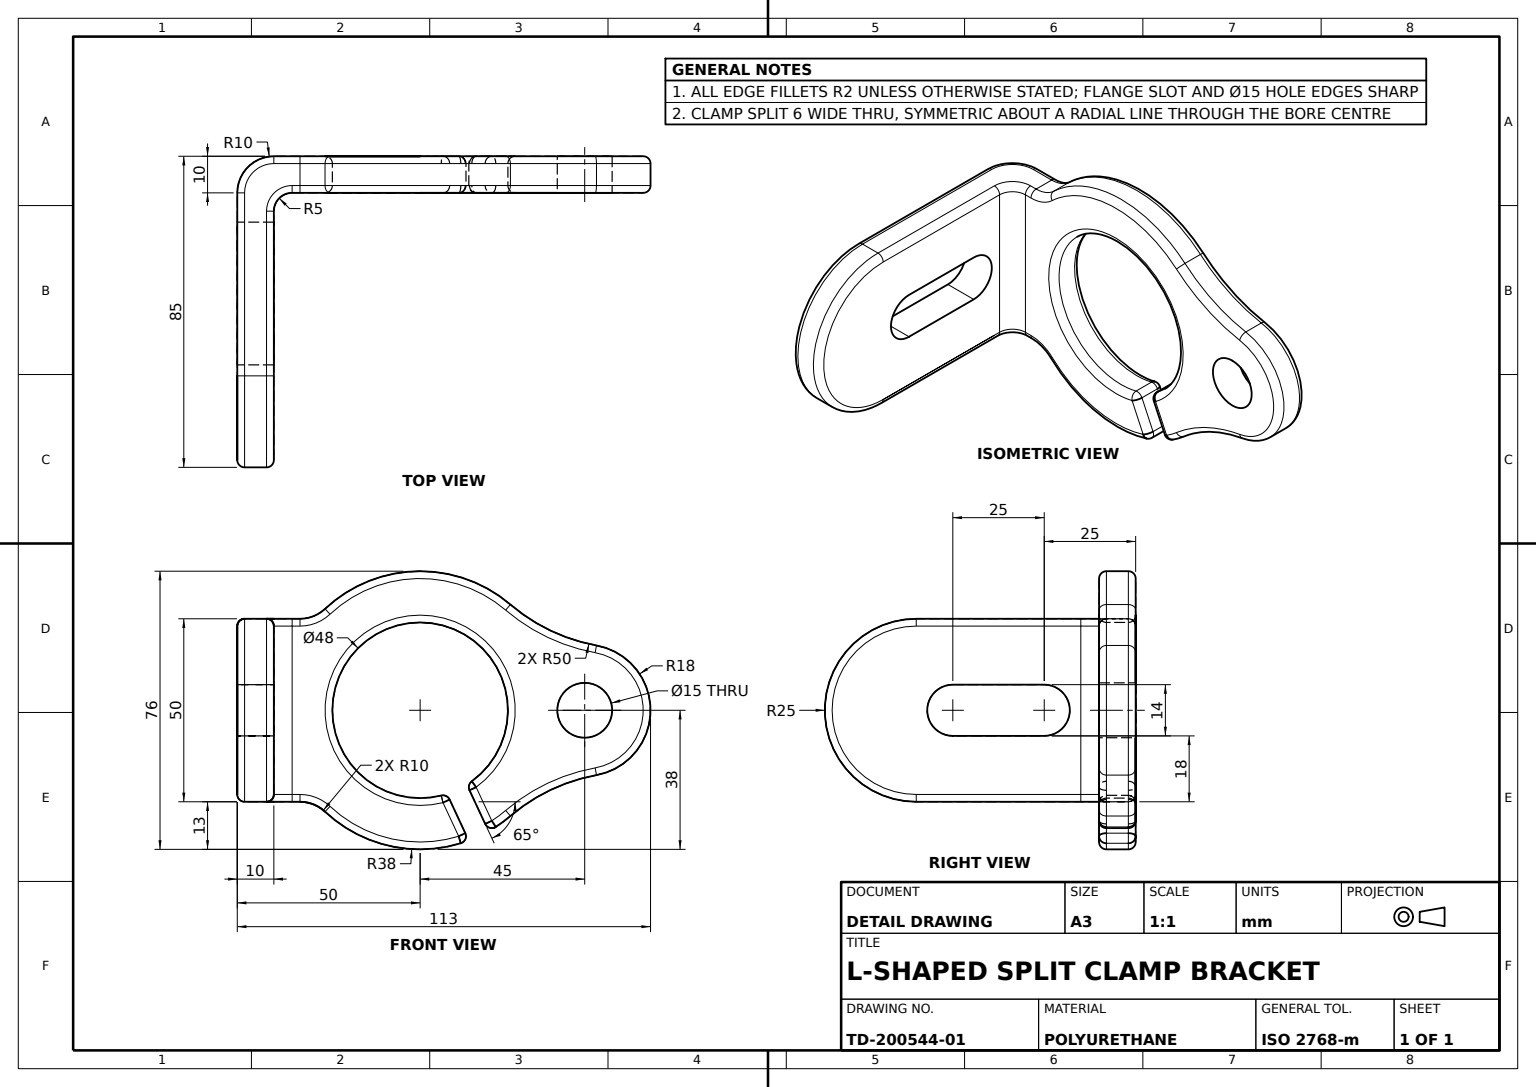
from build123d import *

# Parameters (mm, degrees)
CLAMP_PLATE_SKETCH_R      = 24
CLAMP_PLATE_SKETCH_R_2    = 7.5
CLAMP_RING_PLATE_DEPTH    = 10
SLOTTED_TOP_FLANGE_DEPTH  = 10
CLAMP_SPLIT_CUT_DEPTH     = 141.847435191
FLANGE_BEND_FILLET_R5_R   = 5
PLATE_CORNER_FILLET_R10_R = 10
EDGE_BREAK_FILLETS_R2_R   = 2


with BuildPart() as part:
    # Clamp Plate Sketch → Clamp Ring Plate (new body)
    with BuildSketch(Plane.XY):
        with BuildLine():
            Line((25, 0), (25, -17.151864589))
            ThreePointArc((25, -17.151864589), (25.701702665, -20.83176495), (27.708333333, -23.995226133))
            ThreePointArc((27.708333333, -23.995226133), (37.989682547, -49.114550984), (28.889805354, -74.685606061))
            ThreePointArc((28.889805354, -74.685606061), (21.739686255, -85.712027428), (17.709540124, -98.220588235))
            ThreePointArc((17.709540124, -98.220588235), (0, -113), (-17.709540124, -98.220588235))
            ThreePointArc((-17.709540124, -98.220588235), (-21.739686255, -85.712027428), (-28.889805354, -74.685606061))
            ThreePointArc((-28.889805354, -74.685606061), (-37.989682547, -49.114550984), (-27.708333333, -23.995226133))
            ThreePointArc((-27.708333333, -23.995226133), (-25.701702665, -20.83176495), (-25, -17.151864589))
            Line((-25, -17.151864589), (-25, 0))
            Line((-25, 0), (25, 0))
        make_face()
        with Locations((0, -50)):
            Circle(CLAMP_PLATE_SKETCH_R, mode=Mode.SUBTRACT)
        with Locations((0, -95)):
            Circle(CLAMP_PLATE_SKETCH_R_2, mode=Mode.SUBTRACT)
    extrude(amount=CLAMP_RING_PLATE_DEPTH)

    # Top Flange Sketch → Slotted Top Flange (add)
    with BuildSketch(Plane(origin=(0, 0, 0), x_dir=(1, 0, 0), z_dir=(0, 1, 0))):
        with BuildLine():
            Line((-25, -10), (25, -10))
            Line((25, -10), (25, 50))
            ThreePointArc((25, 50), (0, 75), (-25, 50))
            Line((-25, 50), (-25, -10))
        make_face()
        with BuildLine():
            Line((7, 40), (7, 15))
            ThreePointArc((7, 15), (0, 8), (-7, 15))
            Line((-7, 15), (-7, 40))
            ThreePointArc((-7, 40), (0, 47), (7, 40))
        make_face(mode=Mode.SUBTRACT)
    extrude(amount=-SLOTTED_TOP_FLANGE_DEPTH)

    # Clamp Split Sketch → Clamp Split Cut (cut, through all)
    with BuildSketch(Plane(origin=(0, 0, 0), x_dir=(-1, 0, 0), z_dir=(0, 0, -1))):
        Polygon((-37.744131876, -64.290243987), (-18.548040224, -55.338959443), (-16.012330654, -60.776806166), (-35.208422306, -69.72809071), align=None)
    extrude(amount=-CLAMP_SPLIT_CUT_DEPTH, mode=Mode.SUBTRACT)

    # Flange Bend Fillet R5
    flange_bend_fillet_r5_edges = [part.edges().sort_by_distance(p)[0] for p in [
        (0, -10, 0),
    ]]
    fillet(flange_bend_fillet_r5_edges, radius=FLANGE_BEND_FILLET_R5_R)

    # Plate Corner Fillet R10
    plate_corner_fillet_r10_edges = [part.edges().sort_by_distance(p)[0] for p in [
        (0, 0, 10),
    ]]
    fillet(plate_corner_fillet_r10_edges, radius=PLATE_CORNER_FILLET_R10_R)

    # Edge Break Fillets R2
    edge_break_fillets_r2_edges = [part.edges().sort_by_distance(p)[0] for p in [
        (-25, -16.075932294, 0),
        (25, -10, -27.5),
        (25, -11.464466094, -1.464466094),
        (-37.989682547, -49.114550984, 0),
        (-25, -11.464466094, -1.464466094),
        (-25.701702665, -20.83176495, 0),
        (-25, -13.575932294, 10),
        (-25, 0, -25),
        (-25, -2.928932188, 7.071067812),
        (25, 0, -25),
        (25, -2.928932188, 7.071067812),
        (25, -16.075932294, 0),
        (25.701702665, -20.83176495, 0),
        (31.119955968, -71.807070885, 0),
        (21.739686255, -85.712027428, 10),
        (21.739686255, -85.712027428, 0),
        (0, -113, 0),
        (-21.739686255, -85.712027428, 0),
        (31.119955968, -71.807070885, 10),
        (25.701702665, -20.83176495, 10),
        (25, -13.575932294, 10),
        (-25.701702665, -20.83176495, 10),
        (-37.989682547, -49.114550984, 10),
        (-25, -10, -27.5),
        (0, 0, -75),
        (0, -10, -75),
        (-21.739686255, -85.712027428, 10),
        (-21.751386889, -39.857161718, 10),
        (-21.751386889, -39.857161718, 0),
        (20.312930357, -62.782208742, 5),
        (22.848639927, -57.34436202, 5),
        (37.256095308, -42.517796957, 0),
        (37.256095308, -42.517796957, 10),
        (29.224348471, -60.31740374, 10),
        (35.600057015, -63.29044546, 5),
        (33.064347445, -68.728292182, 5),
        (26.688638901, -65.755250462, 10),
        (26.688638901, -65.755250462, 0),
        (29.224348471, -60.31740374, 0),
        (0, -113, 10),
    ]]
    fillet(edge_break_fillets_r2_edges, radius=EDGE_BREAK_FILLETS_R2_R)


solid = part.part
